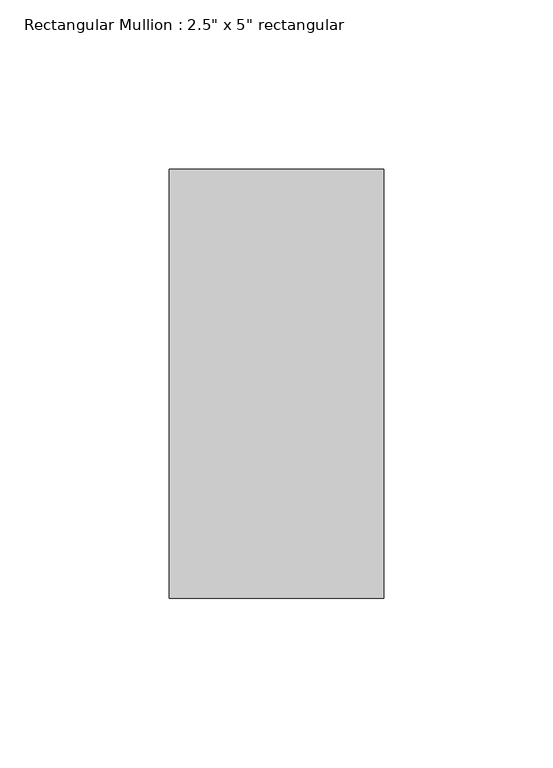
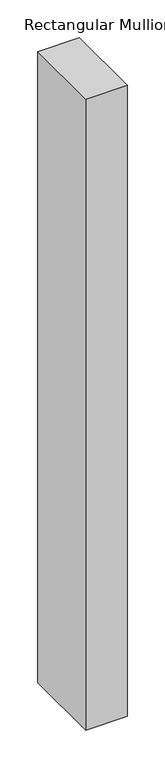
"""IFC4 building model written with IfcOpenShell, lengths in millimetres: member geometry."""

from ifc_helpers import new_model, si_unit, frame, origin, place, context, project, spatial, polyline, outline, extrude, source, transform, mapped, element, save


def member_26f0793c(model_context):
    return source(origin(), model_context, "Body", "SweptSolid", [
        extrude(outline(polyline([(0.0, 63.5), (0.0, -63.5), (-63.5, -63.5), (-63.5, 63.5), (0.0, 63.5)])), frame((0.0, 0.0, -1020.2857817), z_axis=(0.0, 0.0, 1.0), x_axis=(1.0, 0.0, 0.0)), (0.0, 0.0, 1.0), 1020.2857817),
    ])


if __name__ == "__main__":
    model = new_model("IFC4")
    model_context = context("Model", 3, world=origin())
    ifc_project = project(units=[si_unit("LENGTHUNIT", "METRE", prefix="MILLI")], contexts=[model_context])
    site = spatial("IfcSite", under=ifc_project)
    building = spatial("IfcBuilding", under=site)
    placement = place(None, origin())
    member_shape = member_26f0793c(model_context)
    element("IfcMember", 1, ObjectType="Rectangular Mullion : 2.5\" x 5\" rectangular", at=placement, inside=building, context=model_context, shape_type="MappedRepresentation", body=[
        mapped(member_shape, transform((0.0, 0.0, 0.0), x_axis=(1.0, 0.0, 0.0), y_axis=(0.0, 1.0, 0.0), z_axis=(0.0, 0.0, 1.0))),
    ])
    save(model, "model.ifc")

# Revit data of these elements
# Type "Rectangular Mullion : 2.5\" x 5\" rectangular"
#   built-in parameter 1007304 = 0.416667 (stored number, unit not read)
#   built-in parameter 1007301 = 0.104167 (stored number, unit not read)
#   built-in parameter 1007300 = 0.104167 (stored number, unit not read)
# Element 1 (IfcMember, "Rectangular Mullion : 2.5\" x 5\" rectangular")
#   Materials on its faces: "Aluminum"
# Materials
#   "Aluminum": class "Metal", colour RGB 247 247 247, transparency 0, Description = "Aluminum 6061", Cost = 0
